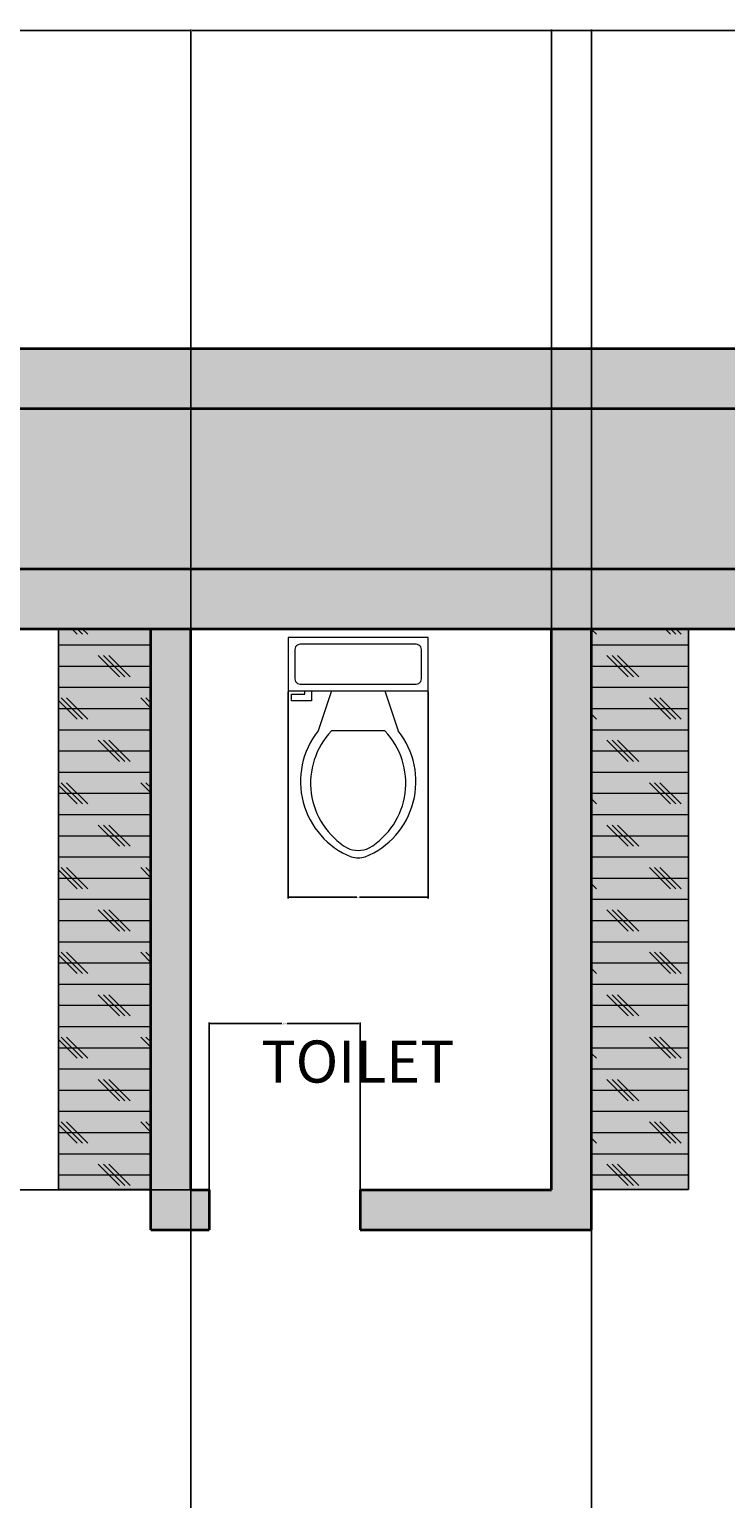
# Model space of a CAD drawing. Units: inches. Extents: x 2549 to 3108, y 1683 to 2362.
# Tile 21 of 30: x 2788 to 2893, y 2142 to 2362. Entities that reach past the tile are written whole.
import ezdxf

# ---------------------------------------------------------------- set-up
doc = ezdxf.new("R2010")
doc.units = ezdxf.units.IN
for name, color, linetype, lineweight in [('A-ANNO-DIMS', 2, 'Continuous', 18), ('A-AREA-IDEN', 7, 'Continuous', 18), ('A-FLOR-CASE', 8, 'Continuous', 25), ('A-FLOR-CASE-PATT', 42, 'Continuous', 13), ('A-FLOR-FIXT', 9, 'Continuous', 18), ('A-FURN-PATT', 9, 'Continuous', 13), ('A-WALL', 7, 'Continuous', 35), ('A-WALL-PATT', 89, 'Continuous', 13), ('C-PROP', 7, 'Continuous', 35)]:
    doc.layers.add(name, color=color, linetype=linetype, lineweight=lineweight)
for name, color, linetype, lineweight, true_color in [('C-PKNG-VEHI-PATT', 251, 'Continuous', 13, 0x636466), ('C-PROP-PATT', 252, 'Continuous', 13, 0x939598), ('C-PVMT-PATT', 9, 'Continuous', 13, 0xc7c8ca)]:
    doc.layers.add(name, color=color, linetype=linetype, lineweight=lineweight, true_color=true_color)
doc.styles.get("Standard").update_dxf_attribs({"font": 'arial.ttf'})
doc.dimstyles.get("Standard").update_dxf_attribs({"dimtxt": 0.18, "dimasz": 0.18, "dimexe": 0.18, "dimexo": 0.0625, "dimgap": 0.09, "dimtad": 0, "dimtih": 1, "dimtoh": 1, "dimdec": 4, "dimzin": 0, "dimdsep": 46, "dimtxsty": 'Standard', "dimcen": 0.09, "dimadec": 0, "dimazin": 0, "dimtfac": 1, "dimtdec": 4, "dimtofl": 0, "dimtmove": 0, "dimatfit": 3, "dimfxl": 1, "dimtolj": 1, "dimtzin": 0, "dimarcsym": 0})

# ---------------------------------------------------------------- blocks, each defined once
blk = doc.blocks.new('*U3')
for p, q in [((9.5, -6), (9.5, -2)), ((-10, -8.5), (-8, -8.5)), ((-10, -9.5), (-10, -8.5)), ((-8, -8.5), (-8, -8)), ((-7, -8), (-7, -9.5)), ((-4, -8), (-6, -14)), ((4, -8), (6, -14)), ((-7, -9.5), (-10, -9.5)), ((4, -14), (-4, -14))]:
    blk.add_line(p, q)
blk.add_lwpolyline([(10.5, -8), (10.5, 0), (-10.5, 0), (-10.5, -8)], close=True)
for points in [[(-9.5, -2), (-9.5, -6)], [(8.5, -1), (-8.5, -1)], [(-8.5, -7), (8.5, -7)]]:
    blk.add_lwpolyline(points)
for centre, radius, start, end in [((-8.62, -1.88), 0.884, 81.8699, 188.1301), ((8.62, -1.88), 0.884, 351.8699, 98.1301), ((-8.62, -6.12), 0.884, 171.8699, 278.1301), ((8.62, -6.12), 0.884, 261.8699, 8.1301), ((3.52, -21.58), 12.17, 141.4691, 247.9714), ((4.2, -21.82), 11.33, 136.3677, 238.9468), ((-3.52, -21.58), 12.17, 292.0284, 38.5307), ((-4.2, -21.82), 11.33, 301.053, 43.6321), ((0, -27.88), 4, 245.7318, 294.2682), ((0, -29), 4, 254.8605, 285.1395)]:
    blk.add_arc(centre, radius, start, end)
blk = doc.blocks.new('*D27')
at = {"layer": 'A-ANNO-DIMS', "color": 0, "lineweight": -2, "transparency": 16777216}
for p, q in [((2629.64, 2281.59), (2629.64, 2362.32)), ((2629.82, 2362.14), (2720.86, 2362.14)), ((2812.46, 2362.14), (2721.42, 2362.14)), ((2812.64, 2272.59), (2812.64, 2362.32))]:
    blk.add_line(p, q, dxfattribs=at)
at = {"layer": 'A-ANNO-DIMS', "color": 0, "transparency": 16777216}
for points in [[(2629.82, 2362.17), (2629.82, 2362.11), (2629.64, 2362.14)], [(2812.46, 2362.17), (2812.46, 2362.11), (2812.64, 2362.14)]]:
    blk.add_solid(points, dxfattribs=at)
at = {"layer": 'Defpoints', "color": 0, "transparency": 16777216}
for p in [(2812.64, 2362.14), (2629.64, 2281.52), (2812.64, 2272.52)]:
    blk.add_point(p, dxfattribs=at)
at = {"layer": 'A-ANNO-DIMS', "color": 0, "transparency": 16777216, "insert": (2721.14, 2362.14), "char_height": 0.18, "attachment_point": 5}
blk.add_mtext('\\A1;183', dxfattribs=at)
blk = doc.blocks.new('*D28')
at = {"layer": 'A-ANNO-DIMS', "color": 0, "lineweight": -2, "transparency": 16777216}
for p, q in [((2812.64, 2272.59), (2812.64, 2362.32)), ((2812.82, 2362.14), (2839.42, 2362.14)), ((2866.46, 2362.14), (2839.86, 2362.14)), ((2866.64, 2272.59), (2866.64, 2362.32))]:
    blk.add_line(p, q, dxfattribs=at)
at = {"layer": 'A-ANNO-DIMS', "color": 0, "transparency": 16777216}
for points in [[(2812.82, 2362.17), (2812.82, 2362.11), (2812.64, 2362.14)], [(2866.46, 2362.17), (2866.46, 2362.11), (2866.64, 2362.14)]]:
    blk.add_solid(points, dxfattribs=at)
at = {"layer": 'Defpoints', "color": 0, "transparency": 16777216}
for p in [(2866.64, 2362.14), (2812.64, 2272.52), (2866.64, 2272.52)]:
    blk.add_point(p, dxfattribs=at)
at = {"layer": 'A-ANNO-DIMS', "color": 0, "transparency": 16777216, "insert": (2839.64, 2362.14), "char_height": 0.18, "attachment_point": 5}
blk.add_mtext('\\A1;54', dxfattribs=at)
blk = doc.blocks.new('*D29')
at = {"layer": 'A-ANNO-DIMS', "color": 0, "lineweight": -2, "transparency": 16777216}
for p, q in [((2866.64, 2272.59), (2866.64, 2362.32)), ((2866.82, 2362.14), (2954.86, 2362.14)), ((3043.46, 2362.14), (2955.42, 2362.14)), ((3043.64, 2281.59), (3043.64, 2362.32))]:
    blk.add_line(p, q, dxfattribs=at)
at = {"layer": 'A-ANNO-DIMS', "color": 0, "transparency": 16777216}
for points in [[(2866.82, 2362.17), (2866.82, 2362.11), (2866.64, 2362.14)], [(3043.46, 2362.17), (3043.46, 2362.11), (3043.64, 2362.14)]]:
    blk.add_solid(points, dxfattribs=at)
at = {"layer": 'Defpoints', "color": 0, "transparency": 16777216}
for p in [(3043.64, 2362.14), (3043.64, 2281.52), (2866.64, 2272.52)]:
    blk.add_point(p, dxfattribs=at)
at = {"layer": 'A-ANNO-DIMS', "color": 0, "transparency": 16777216, "insert": (2955.14, 2362.14), "char_height": 0.18, "attachment_point": 5}
blk.add_mtext('\\A1;177', dxfattribs=at)
blk = doc.blocks.new('*D37')
at = {"layer": 'A-ANNO-DIMS', "color": 0, "lineweight": -2, "transparency": 16777216}
for p, q in [((2812.58, 2272.52), (2781.56, 2272.52)), ((2781.74, 2272.34), (2781.74, 2230.71)), ((2781.74, 2188.7), (2781.74, 2230.34)), ((2812.58, 2188.52), (2781.56, 2188.52))]:
    blk.add_line(p, q, dxfattribs=at)
at = {"layer": 'A-ANNO-DIMS', "color": 0, "transparency": 16777216}
for points in [[(2781.71, 2272.34), (2781.77, 2272.34), (2781.74, 2272.52)], [(2781.71, 2188.7), (2781.77, 2188.7), (2781.74, 2188.52)]]:
    blk.add_solid(points, dxfattribs=at)
at = {"layer": 'Defpoints', "color": 0, "transparency": 16777216}
for p in [(2781.74, 2272.52), (2812.64, 2272.52), (2812.64, 2188.52)]:
    blk.add_point(p, dxfattribs=at)
at = {"layer": 'A-ANNO-DIMS', "color": 0, "transparency": 16777216, "insert": (2781.74, 2230.52), "char_height": 0.18, "attachment_point": 5}
blk.add_mtext('\\A1;84', dxfattribs=at)
blk = doc.blocks.new('*D38')
at = {"layer": 'A-ANNO-DIMS', "color": 0, "lineweight": -2, "transparency": 16777216}
for p, q in [((2815.36, 2182.59), (2815.36, 2213.6)), ((2815.54, 2213.42), (2826.28, 2213.42)), ((2837.81, 2213.42), (2827.07, 2213.42)), ((2837.99, 2182.59), (2837.99, 2213.6))]:
    blk.add_line(p, q, dxfattribs=at)
at = {"layer": 'A-ANNO-DIMS', "color": 0, "transparency": 16777216}
for points in [[(2815.54, 2213.45), (2815.54, 2213.39), (2815.36, 2213.42)], [(2837.81, 2213.45), (2837.81, 2213.39), (2837.99, 2213.42)]]:
    blk.add_solid(points, dxfattribs=at)
at = {"layer": 'Defpoints', "color": 0, "transparency": 16777216}
for p in [(2837.99, 2213.42), (2815.36, 2182.52), (2837.99, 2182.52)]:
    blk.add_point(p, dxfattribs=at)
at = {"layer": 'A-ANNO-DIMS', "color": 0, "transparency": 16777216, "insert": (2826.68, 2213.42), "char_height": 0.18, "attachment_point": 5}
blk.add_mtext('\\A1;22.63', dxfattribs=at)
blk = doc.blocks.new('*D39')
at = {"layer": 'A-ANNO-DIMS', "color": 0, "lineweight": -2, "transparency": 16777216}
for p, q in [((2827.2, 2263.18), (2827.2, 2232.16)), ((2848.2, 2263.18), (2848.2, 2232.16)), ((2827.38, 2232.34), (2837.5, 2232.34)), ((2848.02, 2232.34), (2837.9, 2232.34))]:
    blk.add_line(p, q, dxfattribs=at)
at = {"layer": 'A-ANNO-DIMS', "color": 0, "transparency": 16777216}
for points in [[(2827.38, 2232.37), (2827.38, 2232.31), (2827.2, 2232.34)], [(2848.02, 2232.37), (2848.02, 2232.31), (2848.2, 2232.34)]]:
    blk.add_solid(points, dxfattribs=at)
at = {"layer": 'Defpoints', "color": 0, "transparency": 16777216}
for p in [(2827.2, 2263.24), (2848.2, 2263.24), (2827.2, 2232.34)]:
    blk.add_point(p, dxfattribs=at)
at = {"layer": 'A-ANNO-DIMS', "color": 0, "transparency": 16777216, "insert": (2837.7, 2232.34), "char_height": 0.18, "attachment_point": 5}
blk.add_mtext('\\A1;21', dxfattribs=at)
blk = doc.blocks.new('*D52')
at = {"layer": 'A-ANNO-DIMS', "color": 0, "lineweight": -2, "transparency": 16777216}
for p, q in [((2812.64, 1891.59), (2812.64, 2362.32)), ((2812.82, 2362.14), (2842.42, 2362.14)), ((2872.46, 2362.14), (2842.86, 2362.14)), ((2872.64, 1891.59), (2872.64, 2362.32))]:
    blk.add_line(p, q, dxfattribs=at)
at = {"layer": 'A-ANNO-DIMS', "color": 0, "transparency": 16777216}
for points in [[(2812.82, 2362.17), (2812.82, 2362.11), (2812.64, 2362.14)], [(2872.46, 2362.17), (2872.46, 2362.11), (2872.64, 2362.14)]]:
    blk.add_solid(points, dxfattribs=at)
at = {"layer": 'Defpoints', "color": 0, "transparency": 16777216}
for p in [(2872.64, 2362.14), (2812.64, 1891.52), (2872.64, 1891.52)]:
    blk.add_point(p, dxfattribs=at)
at = {"layer": 'A-ANNO-DIMS', "color": 0, "transparency": 16777216, "insert": (2842.64, 2362.14), "char_height": 0.18, "attachment_point": 5}
blk.add_mtext('\\A1;60', dxfattribs=at)

msp = doc.modelspace()

# ---------------------------------------------------------------- hatches: boundary and pattern name
at = {"layer": 'A-FLOR-CASE-PATT', "transparency": 33554595}
h = msp.add_hatch(dxfattribs=at)
h.set_pattern_fill('CORK', color=256)
h.set_pattern_definition([(0, (0, 0), (0, 3.175), []), (135, (1.5875, -1.5875), (-6.350003, -6.350003), [4.49013, -4.49013]), (135, (2.381, -1.5875), (-6.350003, -6.350003), [4.49013, -4.49013]), (135, (3.175, -1.5875), (-6.350003, -6.350003), [4.49013, -4.49013])])
h.paths.add_polyline_path([(2806.6427, 2272.5237), (2792.7871, 2272.5237), (2792.7871, 2188.5864), (2806.6427, 2188.5864)])
h.paths.add_polyline_path([(2887.1594, 2272.5237), (2872.6427, 2272.5237), (2872.6427, 2188.5907), (2887.1594, 2188.5907)])
at = {"layer": 'A-FLOR-CASE-PATT', "transparency": 33554488}
h = msp.add_hatch(color=256, dxfattribs=at)
h.dxf.hatch_style = 1
h.paths.add_polyline_path([(2806.6427, 2272.5237), (2792.7871, 2272.5237), (2792.7871, 2188.5864), (2806.6427, 2188.5864)])
h.paths.add_polyline_path([(2887.1594, 2272.5237), (2872.6427, 2272.5237), (2872.6427, 2188.5907), (2887.1594, 2188.5907)])
at = {"layer": 'A-FURN-PATT', "transparency": 33554567}
h = msp.add_hatch(color=256, dxfattribs=at)
h.dxf.hatch_style = 1
h.paths.add_polyline_path([(2708.7147, 2271.6737), (2675.2813, 2271.6737), (2675.2813, 2262.0404), (2708.7147, 2262.0404)])
h.paths.add_polyline_path([(2980.8246, 2271.6737), (2947.3913, 2271.6737), (2947.3913, 2262.0404), (2980.8246, 2262.0404)])
h.paths.add_polyline_path([(2748.8496, 2101.6383), (2798.148, 2101.6383), (2798.148, 2111.4248), (2748.8496, 2111.4248)], flags=9)
h.paths.add_polyline_path([(2685.2081, 2101.489), (2719.3253, 2101.489), (2719.3253, 2111.2819), (2685.2081, 2111.2819)], flags=9)
h.paths.add_polyline_path([(2814.6852, 1907.1328), (2847.8384, 1907.1328), (2847.8384, 1916.9258), (2814.6852, 1916.9258)], flags=9)
h.paths.add_polyline_path([(2814.3906, 1835.5864), (2848.0172, 1835.5864), (2848.0172, 1845.3794), (2814.3906, 1845.3794)], flags=9)
h.paths.add_polyline_path([(2800.5245, 1759.1674), (2853.7435, 1759.1674), (2853.7435, 1768.954), (2800.5245, 1768.954)], flags=9)
h.paths.add_polyline_path([(2972.4611, 1807.3305), (3015.3943, 1807.3305), (3015.3943, 1817.117), (2972.4611, 1817.117)], flags=9)
h.paths.add_polyline_path([(2902.3327, 1888.6731), (2937.9131, 1888.6731), (2937.9131, 1898.4661), (2902.3327, 1898.4661)], flags=9)
h.paths.add_polyline_path([(2712.1779, 1878.9039), (2754.1257, 1878.9039), (2754.1257, 1888.6904), (2712.1779, 1888.6904)], flags=9)
h.paths.add_polyline_path([(2614.0056, 2012.812), (2650.0251, 2012.812), (2650.0251, 2022.4371), (2614.0056, 2022.4371)], flags=9)
h.paths.add_polyline_path([(2713.3129, 2003.1645), (2747.4237, 2003.1645), (2747.4237, 2012.951), (2713.3129, 2012.951)], flags=9)
h.paths.add_polyline_path([(2950.1379, 2001.6934), (2982.2992, 2001.6934), (2982.2992, 2011.48), (2950.1379, 2011.48)], flags=9)
h.paths.add_polyline_path([(2940.864, 2238.5537), (2997.5066, 2238.5537), (2997.5066, 2248.3466), (2940.864, 2248.3466)], flags=9)
h.paths.add_polyline_path([(2821.5457, 2202.8348), (2855.663, 2202.8348), (2855.663, 2212.6278), (2821.5457, 2212.6278)], flags=9)
h.paths.add_polyline_path([(2661.8026, 2238.6249), (2718.4451, 2238.6249), (2718.4451, 2248.4179), (2661.8026, 2248.4179)], flags=9)
h = msp.add_hatch(color=256, dxfattribs=at)
h.dxf.hatch_style = 1
h.paths.add_polyline_path([(2906.5064, 1905.2148), (2905.2584, 1904.3827), (2907.0611, 1900.7772), (2908.3092, 1901.6092)])
h.paths.add_polyline_path([(2936.522, 1914.8044), (2935.2739, 1915.6364), (2932.6391, 1912.5856), (2933.8871, 1911.7535)])
h.paths.add_polyline_path([(2950.2508, 1905.6518), (2949.0027, 1906.4839), (2947.1999, 1902.8783), (2948.448, 1902.0463)])
h.paths.add_polyline_path([(2958.5713, 1918.1326), (2956.9072, 1919.242), (2952.4696, 1908.98, 1.38742744), (2954.9657, 1907.3159)])
h.paths.add_polyline_path([(2945.2585, 1927.0078), (2943.5944, 1928.1172), (2934.9965, 1920.6287, 1.38742744), (2937.4927, 1918.9646)])
h.paths.add_polyline_path([(2748.8496, 2101.6383), (2798.148, 2101.6383), (2798.148, 2111.4248), (2748.8496, 2111.4248)], flags=9)
h.paths.add_polyline_path([(2685.2081, 2101.489), (2719.3253, 2101.489), (2719.3253, 2111.2819), (2685.2081, 2111.2819)], flags=9)
h.paths.add_polyline_path([(2814.6852, 1907.1328), (2847.8384, 1907.1328), (2847.8384, 1916.9258), (2814.6852, 1916.9258)], flags=9)
h.paths.add_polyline_path([(2814.3906, 1835.5864), (2848.0172, 1835.5864), (2848.0172, 1845.3794), (2814.3906, 1845.3794)], flags=9)
h.paths.add_polyline_path([(2800.5245, 1759.1674), (2853.7435, 1759.1674), (2853.7435, 1768.954), (2800.5245, 1768.954)], flags=9)
h.paths.add_polyline_path([(2972.4611, 1807.3305), (3015.3943, 1807.3305), (3015.3943, 1817.117), (2972.4611, 1817.117)], flags=9)
h.paths.add_polyline_path([(2902.3327, 1888.6731), (2937.9131, 1888.6731), (2937.9131, 1898.4661), (2902.3327, 1898.4661)], flags=9)
h.paths.add_polyline_path([(2712.1779, 1878.9039), (2754.1257, 1878.9039), (2754.1257, 1888.6904), (2712.1779, 1888.6904)], flags=9)
h.paths.add_polyline_path([(2614.0056, 2012.812), (2650.0251, 2012.812), (2650.0251, 2022.4371), (2614.0056, 2022.4371)], flags=9)
h.paths.add_polyline_path([(2713.3129, 2003.1645), (2747.4237, 2003.1645), (2747.4237, 2012.951), (2713.3129, 2012.951)], flags=9)
h.paths.add_polyline_path([(2950.1379, 2001.6934), (2982.2992, 2001.6934), (2982.2992, 2011.48), (2950.1379, 2011.48)], flags=9)
h.paths.add_polyline_path([(2940.864, 2238.5537), (2997.5066, 2238.5537), (2997.5066, 2248.3466), (2940.864, 2248.3466)], flags=9)
h.paths.add_polyline_path([(2821.5457, 2202.8348), (2855.663, 2202.8348), (2855.663, 2212.6278), (2821.5457, 2212.6278)], flags=9)
h.paths.add_polyline_path([(2661.8026, 2238.6249), (2718.4451, 2238.6249), (2718.4451, 2248.4179), (2661.8026, 2248.4179)], flags=9)
at = {"layer": 'A-WALL-PATT'}
h = msp.add_hatch(color=256, dxfattribs=at)
h.dxf.hatch_style = 1
h.paths.add_polyline_path([(2638.6427, 2272.5237), (3034.6427, 2272.5237), (3034.6427, 1936.5237), (3043.6427, 1936.5237), (3043.6427, 2281.5237), (2629.6427, 2281.5237), (2629.6427, 2074.5237), (2812.6427, 2074.5237), (2812.6427, 2140.5237), (2785.7177, 2140.5237), (2785.7177, 2134.5237), (2806.6427, 2134.5237), (2806.6427, 2080.5237), (2638.6427, 2080.5237)])
h.paths.add_polyline_path([(2638.6427, 1972.5237), (2662.6427, 1972.5237), (2662.6427, 2041.0557), (2653.6427, 2041.0557), (2653.6427, 1978.5237), (2629.6427, 1978.5237), (2629.6427, 1795.5237), (2662.6427, 1795.5237), (2881.6427, 1795.5237), (2881.6427, 1936.5237), (2965.9351, 1936.5237), (2965.9351, 1974.5439), (2959.9351, 1974.5439), (2959.9351, 1945.5237), (2881.6427, 1945.5237), (2872.6427, 1945.5237), (2872.6427, 1804.5237), (2662.6427, 1804.5237), (2638.6427, 1804.5237)])
h = msp.add_hatch(color=256, dxfattribs=at)
h.dxf.hatch_style = 1
h.paths.add_polyline_path([(2812.6427, 2272.5237), (2806.6427, 2272.5237), (2806.6427, 2182.5237), (2815.3646, 2182.5237), (2815.3646, 2188.5237), (2812.6427, 2188.5237)])
h.paths.add_polyline_path([(2872.6427, 2272.5237), (2866.6427, 2272.5237), (2866.6427, 2188.5237), (2837.9934, 2188.5237), (2837.9934, 2182.5237), (2872.6427, 2182.5237)])
h.paths.add_polyline_path([(3034.6427, 2140.5237), (2866.6427, 2140.5237), (2866.6427, 2134.5237), (3034.6427, 2134.5237)])
at = {"layer": 'C-PKNG-VEHI-PATT'}
h = msp.add_hatch(color=256, dxfattribs=at)
h.dxf.hatch_style = 1
edge = h.paths.add_edge_path()
edge.add_ellipse((2935.7258, 1791.964), major_axis=(-50.66, 0), ratio=0.84230387, start_angle=248.165046, end_angle=265.722579)
edge.add_line((2938.911, 1834.5507), (2925.8653, 1834.5507))
edge.add_ellipse((2929.0505, 1791.964), major_axis=(50.66, 0), ratio=0.84230387, start_angle=94.277421, end_angle=111.834954)
edge.add_line((2912.8508, 1832.3947), (2914.2044, 1822.2495))
edge.add_ellipse((2930.6538, 1783.1023), major_axis=(-49.3014, 0), ratio=0.84230387, start_angle=-85.12993, end_angle=-67.208085, ccw=False)
edge.add_line((2927.1247, 1824.5225), (2937.6516, 1824.5225))
edge.add_ellipse((2934.1225, 1783.1023), major_axis=(49.3014, 0), ratio=0.84230387, start_angle=67.208085, end_angle=85.12993, ccw=False)
edge.add_line((2950.5719, 1822.2495), (2951.9255, 1832.3947))
edge = h.paths.add_edge_path()
edge.add_ellipse((2903.4793, 1857.3351), major_axis=(-34.7979, 0), ratio=0.84230387, start_angle=180, end_angle=209.43857)
edge.add_ellipse((2961.297, 1857.3351), major_axis=(34.7979, 0), ratio=0.84230387, start_angle=150.56143, end_angle=180)
edge.add_line((2926.4991, 1857.3351), (2926.4991, 1843.7609))
edge.add_ellipse((2924.1251, 1844.3143), major_axis=(-0.2209, 3.9278), ratio=0.60383358, start_angle=89.002014, end_angle=253.657408, ccw=False)
edge.add_line((2921.7512, 1844.2222), (2921.7512, 1853.3975))
edge.add_line((2921.7512, 1853.3975), (2925.269, 1855.8484))
edge.add_ellipse((2925.4782, 1855.4931), major_axis=(0.4584, 0), ratio=0.84230387, start_angle=90, end_angle=134.480211, ccw=False)
edge.add_line((2925.4782, 1855.8792), (2926.4991, 1855.8792))
edge.add_line((2926.4991, 1855.8792), (2926.4991, 1857.3351))
edge.add_ellipse((2961.297, 1857.3351), major_axis=(34.7979, 0), ratio=0.84230387, start_angle=150.56143, end_angle=180, ccw=False)
edge.add_line((2932.3882, 1873.6501), (2932.3882, 1875.7801))
edge.add_ellipse((2932.3882, 1875.3939), major_axis=(0.4584, 0), ratio=0.84230387, start_angle=90, end_angle=127.93313)
edge.add_line((2932.1366, 1875.7167), (2928.5915, 1873.7564))
edge.add_ellipse((2899.9271, 2002.4692), major_axis=(155.4756, 0), ratio=0.84230387, start_angle=-80.743434, end_angle=-77.445067, ccw=False)
edge.add_ellipse((2949.4402, 1715.2151), major_axis=(-189.1422, 0), ratio=0.84230387, start_angle=-79.790461, end_angle=-77.555373)
edge.add_ellipse((3300.3614, 1852.5642), major_axis=(-386.1662, 0), ratio=0.84230387, start_angle=-2.863715, end_angle=2.198541)
edge.add_ellipse((2929.0505, 1792.5159), major_axis=(-55.6192, 0), ratio=0.84230387, start_angle=-85.917589, end_angle=-72.280047, ccw=False)
edge.add_line((2925.7129, 1839.2798), (2939.0634, 1839.2798))
edge.add_ellipse((2935.7258, 1792.5159), major_axis=(55.6192, 0), ratio=0.84230387, start_angle=72.280047, end_angle=85.917589, ccw=False)
edge.add_ellipse((2564.4149, 1852.5642), major_axis=(-386.1662, 0), ratio=0.84230387, start_angle=177.801459, end_angle=182.863715)
edge.add_ellipse((2915.3361, 1715.2151), major_axis=(189.1422, 0), ratio=0.84230387, start_angle=77.555373, end_angle=79.790461)
edge.add_ellipse((2964.8492, 2002.4692), major_axis=(-155.4756, 0), ratio=0.84230387, start_angle=77.445067, end_angle=80.743434, ccw=False)
edge.add_line((2936.1848, 1873.7564), (2932.6397, 1875.7167))
edge.add_ellipse((2932.3882, 1875.3939), major_axis=(0.4584, 0), ratio=0.84230387, start_angle=52.06687, end_angle=90)
edge.add_line((2932.3882, 1875.7801), (2932.3882, 1873.6501))
edge.add_ellipse((2903.4793, 1857.3351), major_axis=(-34.7979, 0), ratio=0.84230387, start_angle=180, end_angle=209.43857, ccw=False)
edge.add_line((2938.2772, 1857.3351), (2938.2772, 1855.8792))
edge.add_line((2938.2772, 1855.8792), (2939.4059, 1855.8792))
edge.add_ellipse((2939.2981, 1855.4931), major_axis=(-0.4584, 0), ratio=0.84230387, start_angle=225.519789, end_angle=270, ccw=False)
edge.add_line((2939.5903, 1855.7906), (2943.0251, 1853.3975))
edge.add_line((2943.0251, 1853.3975), (2943.0251, 1844.2222))
edge.add_ellipse((2940.6512, 1844.3143), major_axis=(0.2209, 3.9278), ratio=0.60383358, start_angle=106.342592, end_angle=270.997986, ccw=False)
edge.add_line((2938.2772, 1843.7609), (2938.2772, 1857.3351))
edge = h.paths.add_edge_path()
edge.add_ellipse((2932.3882, 1865.1973), major_axis=(91.081, 0), ratio=0.84230387, start_angle=256.401865, end_angle=283.598135, ccw=False)
edge.add_line((2914.2044, 1790.0239), (2914.2044, 1778.3622))
edge.add_ellipse((2932.3882, 1853.5356), major_axis=(91.081, 0), ratio=0.84230387, start_angle=256.401865, end_angle=283.598135)
edge.add_line((2950.5719, 1778.3622), (2950.5719, 1790.0239))
edge = h.paths.add_edge_path()
edge.add_ellipse((2948.7383, 1772.3145), major_axis=(1.8336, 0), ratio=0.84230387, start_angle=0, end_angle=90)
edge.add_line((2948.7383, 1773.859), (2916.038, 1773.859))
edge.add_ellipse((2916.038, 1772.3145), major_axis=(1.8336, 0), ratio=0.84230387, start_angle=90, end_angle=180)
edge.add_line((2914.2044, 1772.3145), (2914.2044, 1760.2558))
edge.add_line((2914.2044, 1760.2558), (2950.5719, 1760.2558))
edge.add_line((2950.5719, 1760.2558), (2950.5719, 1772.3145))
h.paths.add_polyline_path([(2748.8496, 2101.6383), (2798.148, 2101.6383), (2798.148, 2111.4248), (2748.8496, 2111.4248)], flags=9)
h.paths.add_polyline_path([(2685.2081, 2101.489), (2719.3253, 2101.489), (2719.3253, 2111.2819), (2685.2081, 2111.2819)], flags=9)
h.paths.add_polyline_path([(2814.6852, 1907.1328), (2847.8384, 1907.1328), (2847.8384, 1916.9258), (2814.6852, 1916.9258)], flags=9)
h.paths.add_polyline_path([(2814.3906, 1835.5864), (2848.0172, 1835.5864), (2848.0172, 1845.3794), (2814.3906, 1845.3794)], flags=9)
h.paths.add_polyline_path([(2800.5245, 1759.1674), (2853.7435, 1759.1674), (2853.7435, 1768.954), (2800.5245, 1768.954)], flags=9)
h.paths.add_polyline_path([(2972.4611, 1807.3305), (3015.3943, 1807.3305), (3015.3943, 1817.117), (2972.4611, 1817.117)], flags=9)
h.paths.add_polyline_path([(2902.3327, 1888.6731), (2937.9131, 1888.6731), (2937.9131, 1898.4661), (2902.3327, 1898.4661)], flags=9)
h.paths.add_polyline_path([(2712.1779, 1878.9039), (2754.1257, 1878.9039), (2754.1257, 1888.6904), (2712.1779, 1888.6904)], flags=9)
h.paths.add_polyline_path([(2614.0056, 2012.812), (2650.0251, 2012.812), (2650.0251, 2022.4371), (2614.0056, 2022.4371)], flags=9)
h.paths.add_polyline_path([(2713.3129, 2003.1645), (2747.4237, 2003.1645), (2747.4237, 2012.951), (2713.3129, 2012.951)], flags=9)
h.paths.add_polyline_path([(2950.1379, 2001.6934), (2982.2992, 2001.6934), (2982.2992, 2011.48), (2950.1379, 2011.48)], flags=9)
h.paths.add_polyline_path([(2940.864, 2238.5537), (2997.5066, 2238.5537), (2997.5066, 2248.3466), (2940.864, 2248.3466)], flags=9)
h.paths.add_polyline_path([(2821.5457, 2202.8348), (2855.663, 2202.8348), (2855.663, 2212.6278), (2821.5457, 2212.6278)], flags=9)
h.paths.add_polyline_path([(2661.8026, 2238.6249), (2718.4451, 2238.6249), (2718.4451, 2248.4179), (2661.8026, 2248.4179)], flags=9)
at = {"layer": 'C-PROP-PATT'}
h = msp.add_hatch(color=256, dxfattribs=at)
h.dxf.hatch_style = 1
h.paths.add_polyline_path([(3076.6427, 2314.5237), (2596.6427, 2314.5237), (2596.6427, 1714.5237), (2881.84, 1714.5237), (2881.84, 1723.5237), (2605.6427, 1723.5237), (2605.6427, 2305.5237), (3067.6427, 2305.5237), (3067.6427, 1723.5237), (3067.6427, 1714.5237), (3076.6427, 1714.5237)])
at = {"layer": 'C-PVMT-PATT'}
h = msp.add_hatch(color=256, dxfattribs=at)
h.dxf.hatch_style = 1
h.paths.add_polyline_path([(3067.6427, 2305.5237), (2605.6427, 2305.5237), (2605.6427, 2074.5237), (2629.6427, 2074.5237), (2629.6427, 2281.5237), (3043.6427, 2281.5237), (3043.6427, 1885.5237), (3043.6427, 1872.8745), (3031.1672, 1872.8745), (3031.1672, 1862.5731), (2995.8054, 1862.5731), (2995.8054, 1872.8745), (2983.1752, 1872.8745), (2983.1752, 1885.5237), (2881.6427, 1885.5237), (2881.6427, 1795.5237), (2751.0977, 1795.5237), (2751.0977, 1761.5237), (2786.1577, 1761.5237), (2786.1577, 1723.5237), (2881.84, 1723.5237), (2881.84, 1714.5237), (3067.6427, 1714.5237), (3067.6427, 1723.5237)])
edge = h.paths.add_edge_path(flags=16)
edge.add_ellipse((2949.4402, 1710.9683), major_axis=(-194.1014, 0), ratio=0.84230387, start_angle=-77.874034, end_angle=-76.219471, ccw=False)
edge.add_ellipse((2949.4402, 1715.2151), major_axis=(-189.1422, 0), ratio=0.84230387, start_angle=-79.790461, end_angle=-77.555373, ccw=False)
edge.add_ellipse((2899.9271, 2002.4692), major_axis=(155.4756, 0), ratio=0.84230387, start_angle=-80.743434, end_angle=-77.445067)
edge.add_line((2928.5915, 1873.7564), (2932.3882, 1875.8558))
edge.add_line((2932.3882, 1875.8558), (2936.1848, 1873.7564))
edge.add_ellipse((2964.8492, 2002.4692), major_axis=(-155.4756, 0), ratio=0.84230387, start_angle=77.445067, end_angle=80.743434)
edge.add_ellipse((2915.3361, 1715.2151), major_axis=(189.1422, 0), ratio=0.84230387, start_angle=77.555373, end_angle=79.790461, ccw=False)
edge.add_ellipse((2915.3361, 1710.9683), major_axis=(-194.1014, 0), ratio=0.84230387, start_angle=256.219471, end_angle=257.874034, ccw=False)
edge.add_ellipse((2628.2871, 1850.2612), major_axis=(-327.2532, 0), ratio=0.84230387, start_angle=182.17995, end_angle=183.650428, ccw=False)
edge.add_ellipse((2955.5637, 1861.9334), major_axis=(-0.9168, 0), ratio=0.84230387, start_angle=180, end_angle=270, ccw=False)
edge.add_line((2956.4805, 1862.3857), (2956.4805, 1846.4866))
edge.add_ellipse((2955.5637, 1846.939), major_axis=(-0.9168, 0), ratio=0.84230387, start_angle=90, end_angle=180, ccw=False)
edge.add_ellipse((-3607.0606, 1835.832), major_axis=(-6562.6242, 0), ratio=0.84230387, start_angle=179.61613322, end_angle=180.09022909, ccw=False)
edge.add_ellipse((2955.5637, 1791.0926), major_axis=(0.9168, 0), ratio=0.84230387, start_angle=0, end_angle=90, ccw=False)
edge.add_line((2956.4805, 1791.545), (2956.4805, 1775.6459))
edge.add_ellipse((2955.5637, 1776.0982), major_axis=(0.9168, 0), ratio=0.84230387, start_angle=270, end_angle=360, ccw=False)
edge.add_ellipse((-3607.0606, 1835.832), major_axis=(-6562.6242, 0), ratio=0.84230387, start_angle=179.3813568, end_angle=179.47172853, ccw=False)
edge.add_ellipse((2954.5907, 1763.8768), major_axis=(-1.3752, 0), ratio=0.84230387, start_angle=179.371763, end_angle=248.464757, ccw=False)
edge.add_ellipse((-3607.519, 1835.832), major_axis=(-6564.0409, 0), ratio=0.842303863, start_angle=179.35344594, end_angle=179.37176282, ccw=False)
edge.add_ellipse((2952.6829, 1761.8002), major_axis=(3.2503, 0), ratio=0.84230387, start_angle=-90, end_angle=-0.646554, ccw=False)
edge.add_line((2952.6829, 1759.0625), (2912.0934, 1759.0625))
edge.add_ellipse((2912.0934, 1761.8002), major_axis=(3.2503, 0), ratio=0.84230387, start_angle=180.646554, end_angle=270, ccw=False)
edge.add_ellipse((9472.2953, 1835.832), major_axis=(-6564.0409, 0), ratio=0.842303871, start_angle=0.62823722, end_angle=0.6465541, ccw=False)
edge.add_ellipse((2910.1856, 1763.8768), major_axis=(1.3752, 0), ratio=0.84230387, start_angle=111.535244, end_angle=180.628237, ccw=False)
edge.add_ellipse((9471.8369, 1835.832), major_axis=(-6562.6242, 0), ratio=0.84230387, start_angle=0.52827147, end_angle=0.6465541, ccw=False)
edge.add_ellipse((2909.2126, 1776.0982), major_axis=(-0.9168, 0), ratio=0.84230387, start_angle=0, end_angle=90, ccw=False)
edge.add_line((2908.2958, 1775.6459), (2908.2958, 1791.545))
edge.add_ellipse((2909.2126, 1791.0926), major_axis=(-0.9168, 0), ratio=0.84230387, start_angle=-90, end_angle=0, ccw=False)
edge.add_ellipse((9471.8369, 1835.832), major_axis=(-6562.6242, 0), ratio=0.84230387, start_angle=-0.09022909, end_angle=0.38386678, ccw=False)
edge.add_ellipse((2909.2126, 1846.939), major_axis=(-0.9168, 0), ratio=0.84230387, start_angle=0, end_angle=90, ccw=False)
edge.add_line((2908.2958, 1846.4866), (2908.2958, 1862.3857))
edge.add_ellipse((2909.2126, 1861.9334), major_axis=(0.9168, 0), ratio=0.84230387, start_angle=90, end_angle=180, ccw=False)
edge.add_ellipse((3236.4892, 1850.2612), major_axis=(327.2532, 0), ratio=0.84230387, start_angle=176.349572, end_angle=177.82005, ccw=False)
edge = h.paths.add_edge_path(flags=0)
edge.add_ellipse((2903.4793, 1857.3351), major_axis=(-34.7979, 0), ratio=0.84230387, start_angle=180, end_angle=209.43857, ccw=False)
edge.add_line((2938.2772, 1857.3351), (2938.2772, 1855.8792))
edge.add_line((2938.2772, 1855.8792), (2939.4631, 1855.8792))
edge.add_line((2939.4631, 1855.8792), (2943.0251, 1853.3975))
edge.add_line((2943.0251, 1853.3975), (2943.0251, 1844.2222))
edge.add_ellipse((2940.6512, 1844.3143), major_axis=(0.2209, 3.9278), ratio=0.60383358, start_angle=106.342592, end_angle=270.997986, ccw=False)
edge.add_line((2938.2772, 1843.7609), (2938.2772, 1857.3351))
edge.add_ellipse((2903.4793, 1857.3351), major_axis=(-34.7979, 0), ratio=0.84230387, start_angle=180, end_angle=209.43857)
edge.add_ellipse((2961.297, 1857.3351), major_axis=(34.7979, 0), ratio=0.84230387, start_angle=150.56143, end_angle=180)
edge.add_line((2926.4991, 1857.3351), (2926.4991, 1843.7609))
edge.add_ellipse((2924.1251, 1844.3143), major_axis=(-0.2209, 3.9278), ratio=0.60383358, start_angle=89.002014, end_angle=253.657408, ccw=False)
edge.add_line((2921.7512, 1844.2222), (2921.7512, 1853.3975))
edge.add_line((2921.7512, 1853.3975), (2925.3132, 1855.8792))
edge.add_line((2925.3132, 1855.8792), (2926.4991, 1855.8792))
edge.add_line((2926.4991, 1855.8792), (2926.4991, 1857.3351))
edge.add_ellipse((2961.297, 1857.3351), major_axis=(34.7979, 0), ratio=0.84230387, start_angle=150.56143, end_angle=180, ccw=False)
edge = h.paths.add_edge_path(flags=0)
edge.add_ellipse((2929.0505, 1791.964), major_axis=(50.66, 0), ratio=0.84230387, start_angle=94.277421, end_angle=111.834954, ccw=False)
edge.add_line((2925.8653, 1834.5507), (2938.911, 1834.5507))
edge.add_ellipse((2935.7258, 1791.964), major_axis=(-50.66, 0), ratio=0.84230387, start_angle=248.165046, end_angle=265.722579, ccw=False)
edge.add_line((2951.9255, 1832.3947), (2950.5719, 1822.2495))
edge.add_ellipse((2934.1225, 1783.1023), major_axis=(49.3014, 0), ratio=0.84230387, start_angle=67.208085, end_angle=85.12993)
edge.add_line((2937.6516, 1824.5225), (2927.1247, 1824.5225))
edge.add_ellipse((2930.6538, 1783.1023), major_axis=(-49.3014, 0), ratio=0.84230387, start_angle=-85.12993, end_angle=-67.208085)
edge.add_line((2914.2044, 1822.2495), (2912.8508, 1832.3947))
edge = h.paths.add_edge_path(flags=0)
edge.add_line((2910.1338, 1829.4651), (2912.6432, 1821.2711))
edge.add_ellipse((5203.7787, 1816.4367), major_axis=(-2291.1426, 0), ratio=0.84230387, start_angle=-0.1208974, end_angle=0.3640763)
edge.add_line((2912.7012, 1801.8782), (2910.3305, 1792.5698))
edge.add_ellipse((9471.8369, 1835.832), major_axis=(-6561.7074, 0), ratio=0.84230387, start_angle=0.05559431, end_angle=0.37776419, ccw=False)
edge = h.paths.add_edge_path(flags=0)
edge.add_ellipse((-3607.0606, 1835.832), major_axis=(6561.7074, 0), ratio=0.84230387, start_angle=-0.37776419, end_angle=-0.05559431, ccw=False)
edge.add_line((2954.4458, 1792.5698), (2952.0751, 1801.8782))
edge.add_ellipse((660.9976, 1816.4367), major_axis=(2291.1426, 0), ratio=0.84230387, start_angle=-0.3640763, end_angle=0.1208974)
edge.add_line((2952.1331, 1821.2711), (2954.6425, 1829.4651))
edge = h.paths.add_edge_path(flags=0)
edge.add_ellipse((2932.3882, 1865.1973), major_axis=(91.081, 0), ratio=0.84230387, start_angle=256.401865, end_angle=283.598135)
edge.add_line((2950.5719, 1790.0239), (2950.5719, 1778.3622))
edge.add_ellipse((2932.3882, 1853.5356), major_axis=(91.081, 0), ratio=0.84230387, start_angle=256.401865, end_angle=283.598135, ccw=False)
edge.add_line((2914.2044, 1778.3622), (2914.2044, 1790.0239))
edge = h.paths.add_edge_path(flags=0)
edge.add_line((2916.038, 1773.859), (2948.7383, 1773.859))
edge.add_ellipse((2948.7383, 1772.3145), major_axis=(1.8336, 0), ratio=0.84230387, start_angle=0, end_angle=90, ccw=False)
edge.add_line((2950.5719, 1772.3145), (2950.5719, 1760.2558))
edge.add_line((2950.5719, 1760.2558), (2914.2044, 1760.2558))
edge.add_line((2914.2044, 1760.2558), (2914.2044, 1772.3145))
edge.add_ellipse((2916.038, 1772.3145), major_axis=(1.8336, 0), ratio=0.84230387, start_angle=90, end_angle=180, ccw=False)
h.paths.add_polyline_path([(2629.6427, 1978.5237), (2605.6427, 1978.5237), (2605.6427, 1723.5237), (2629.6427, 1723.5237), (2629.6427, 1795.5237)], flags=17)
h.paths.add_polyline_path([(2800.5245, 1759.1674), (2853.7435, 1759.1674), (2853.7435, 1768.954), (2800.5245, 1768.954)], flags=24)
h.paths.add_polyline_path([(2972.4611, 1807.3305), (3015.3943, 1807.3305), (3015.3943, 1817.117), (2972.4611, 1817.117)], flags=24)

# ---------------------------------------------------------------- linework, layer by layer
at = {"layer": 'A-FLOR-CASE'}
for p, q in [((2792.7871, 2272.5237), (2792.7871, 2188.5864)), ((2887.1594, 2188.5907), (2887.1594, 2272.5237)), ((2792.7871, 2188.5864), (2806.6427, 2188.5864)), ((2872.6427, 2188.5907), (2887.1594, 2188.5907))]:
    msp.add_line(p, q, dxfattribs=at)
at = {"layer": 'A-WALL'}
for p, q in [((2629.6427, 2281.5237), (3043.6427, 2281.5237)), ((2638.6427, 2272.5237), (3034.6427, 2272.5237)), ((2806.6427, 2182.5237), (2806.6427, 2272.5237)), ((2812.6427, 2188.5237), (2812.6427, 2272.5237)), ((2866.6427, 2188.5237), (2866.6427, 2272.5237)), ((2872.6427, 2182.5237), (2872.6427, 2272.5237)), ((2812.6427, 2188.5237), (2815.3646, 2188.5237)), ((2815.3646, 2188.5237), (2815.3646, 2182.5237)), ((2837.9934, 2188.5237), (2837.9934, 2182.5237)), ((2837.9934, 2188.5237), (2866.6427, 2188.5237)), ((2806.6427, 2182.5237), (2815.3646, 2182.5237)), ((2837.9934, 2182.5237), (2872.6427, 2182.5237))]:
    msp.add_line(p, q, dxfattribs=at)
at = {"layer": 'C-PROP'}
msp.add_lwpolyline([(2596.6427, 2314.5237), (3076.6427, 2314.5237), (3076.6427, 1714.5237), (2596.6427, 1714.5237)], close=True, dxfattribs=at)
msp.add_lwpolyline([(2881.84, 1723.5237), (2605.6427, 1723.5237), (2605.6427, 2305.5237), (3067.6427, 2305.5237), (3067.6427, 1723.5237)], dxfattribs=at)

# ---------------------------------------------------------------- block references
at = {"layer": 'A-FLOR-FIXT'}
msp.add_blockref('*U3', (2837.7005, 2271.2425), dxfattribs=at)

# ---------------------------------------------------------------- texts
at = {"layer": 'A-AREA-IDEN'}
msp.add_text('TOILET', height=6.30916, dxfattribs=at).set_placement((2823.1779, 2204.5746))

# ---------------------------------------------------------------- dimensions: what is measured, and where the dimension line sits
at = {"layer": 'A-ANNO-DIMS'}
for base, p1, p2, override, picture, middle in [((2812.6427, 2362.1425), (2629.6427, 2281.5237), (2812.6427, 2272.5237), {"dimdec": 0, "dimlfac": 1, "dimrnd": 0, "dimzin": 0, "dimdsep": 46, "dimlunit": 2}, '*D27', (2721.1427, 2362.1425)), ((2866.6427, 2362.1425), (2812.6427, 2272.5237), (2866.6427, 2272.5237), {"dimdec": 0, "dimlfac": 1, "dimrnd": 0, "dimzin": 0, "dimdsep": 46, "dimlunit": 2}, '*D28', (2839.6427, 2362.1425)), ((2872.6427, 2362.1425), (2812.6427, 1891.5237), (2872.6427, 1891.5237), {"dimdec": 0, "dimlfac": 1, "dimrnd": 0, "dimzin": 0, "dimdsep": 46, "dimlunit": 2}, '*D52', (2842.6427, 2362.1425)), ((3043.6427, 2362.1425), (2866.6427, 2272.5237), (3043.6427, 2281.5237), {"dimdec": 0, "dimlfac": 1, "dimrnd": 0, "dimzin": 0, "dimdsep": 46, "dimlunit": 2}, '*D29', (2955.1427, 2362.1425)), ((2837.9934, 2213.4237), (2815.3646, 2182.5237), (2837.9934, 2182.5237), {"dimdec": 2, "dimlfac": 1, "dimrnd": 0, "dimzin": 0, "dimdsep": 46, "dimlunit": 2}, '*D38', (2826.679, 2213.4237))]:
    dim = msp.add_linear_dim(base=base, p1=p1, p2=p2, dimstyle='Standard', override=override, dxfattribs=at)
    dim.commit()
    dim.dimension.update_dxf_attribs({"geometry": picture, "text_midpoint": middle})
for base, p1, p2, angle, picture, middle in [((2781.7427, 2272.5237), (2812.6427, 2188.5237), (2812.6427, 2272.5237), 90, '*D37', (2781.7427, 2230.5237)), ((2827.2005, 2232.3425), (2848.2005, 2263.2425), (2827.2005, 2263.2425), 180, '*D39', (2837.7005, 2232.3425))]:
    dim = msp.add_linear_dim(base=base, p1=p1, p2=p2, angle=angle, dimstyle='Standard', override={"dimdec": 0, "dimlfac": 1, "dimrnd": 0, "dimzin": 0, "dimdsep": 46, "dimlunit": 2}, dxfattribs=at)
    dim.commit()
    dim.dimension.update_dxf_attribs({"geometry": picture, "text_midpoint": middle})

doc.saveas('drawing.dxf')
